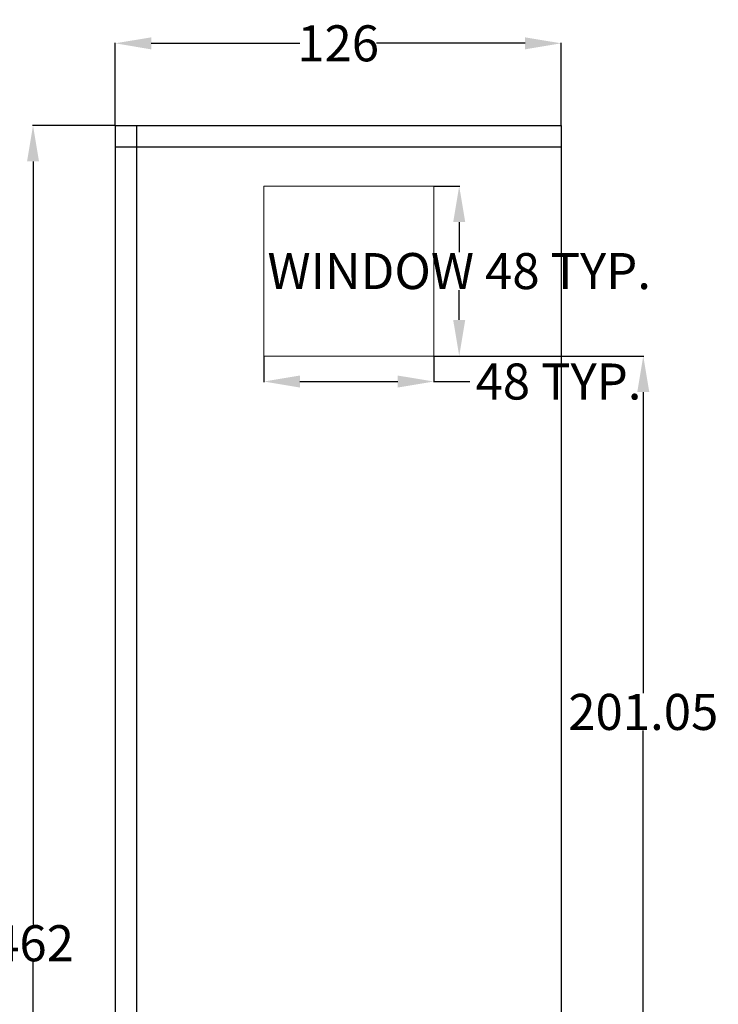
# Model space of a CAD drawing. Units: inches. Extents: x -107 to 647, y -210 to 500.
# Tile 7 of 7: x 450 to 647, y 216 to 494. Entities that reach past the tile are written whole.
import ezdxf

# ---------------------------------------------------------------- set-up
doc = ezdxf.new("R2010")
doc.units = ezdxf.units.IN
doc.header["$MEASUREMENT"] = 0
for name, color, linetype, lineweight in [('A-ANNO-DIMS', 2, 'Continuous', 18), ('A-ELEV', 30, 'Continuous', 25), ('A-ELEV-GLAZ', 4, 'Continuous', 18)]:
    doc.layers.add(name, color=color, linetype=linetype, lineweight=lineweight)
doc.styles.get("Standard").update_dxf_attribs({"font": 'arial.ttf'})
doc.dimstyles.get("Standard").update_dxf_attribs({"dimtxt": 10.18, "dimasz": 10.18, "dimexe": 0.18, "dimexo": 0.0625, "dimgap": 0.09, "dimtad": 0, "dimtih": 1, "dimtoh": 1, "dimdec": 0, "dimzin": 0, "dimdsep": 46, "dimlunit": 3, "dimtxsty": 'Standard', "dimcen": 0.09, "dimadec": 0, "dimazin": 0, "dimtfac": 1, "dimtdec": 0, "dimtofl": 0, "dimtmove": 0, "dimatfit": 3, "dimfxl": 1, "dimtolj": 1, "dimtzin": 0, "dimarcsym": 0})

# ---------------------------------------------------------------- blocks, each defined once
blk = doc.blocks.new('WINDOW-ELEV-48X48IN')
blk.add_lwpolyline([(0, 48), (48, 48), (48, 0), (0, 0)], close=True)
blk = doc.blocks.new('*D42')
at = {"layer": 'A-ANNO-DIMS', "color": 0, "lineweight": -2, "transparency": 16777216}
for p, q in [((566.81, 447.2), (574.13, 447.2)), ((573.95, 437.02), (573.95, 428.55)), ((573.95, 409.38), (573.95, 417.84)), ((566.81, 399.2), (574.13, 399.2))]:
    blk.add_line(p, q, dxfattribs=at)
at = {"layer": 'A-ANNO-DIMS', "color": 0, "transparency": 16777216}
for points in [[(572.25, 437.02), (575.65, 437.02), (573.95, 447.2)], [(572.25, 409.38), (575.65, 409.38), (573.95, 399.2)]]:
    blk.add_solid(points, dxfattribs=at)
at = {"layer": 'Defpoints', "color": 0, "transparency": 16777216}
for p in [(566.75, 447.2), (573.95, 447.2), (566.75, 399.2)]:
    blk.add_point(p, dxfattribs=at)
at = {"layer": 'A-ANNO-DIMS', "color": 0, "transparency": 16777216, "insert": (573.95, 423.2), "char_height": 10.18, "attachment_point": 5}
blk.add_mtext('\\A1;WINDOW 48 TYP.', dxfattribs=at)
blk = doc.blocks.new('*D43')
at = {"layer": 'A-ANNO-DIMS', "color": 0, "lineweight": -2, "transparency": 16777216}
for p, q in [((518.75, 399.14), (518.75, 391.82)), ((566.75, 399.14), (566.75, 391.82)), ((528.93, 392), (556.57, 392)), ((566.75, 392), (576.93, 392))]:
    blk.add_line(p, q, dxfattribs=at)
at = {"layer": 'A-ANNO-DIMS', "color": 0, "transparency": 16777216}
for points in [[(528.93, 393.69), (528.93, 390.3), (518.75, 392)], [(556.57, 393.69), (556.57, 390.3), (566.75, 392)]]:
    blk.add_solid(points, dxfattribs=at)
at = {"layer": 'Defpoints', "color": 0, "transparency": 16777216}
for p in [(518.75, 399.2), (566.75, 399.2), (566.75, 392)]:
    blk.add_point(p, dxfattribs=at)
at = {"layer": 'A-ANNO-DIMS', "color": 0, "transparency": 16777216, "insert": (602, 392), "char_height": 10.18, "attachment_point": 5}
blk.add_mtext('\\A1;48 TYP.', dxfattribs=at)
blk = doc.blocks.new('*D98')
at = {"layer": 'A-ANNO-DIMS', "color": 0, "lineweight": -2, "transparency": 16777216}
for p, q in [((476.69, 464.33), (453.37, 464.33)), ((453.55, 454.15), (453.55, 238.61)), ((453.55, 12.51), (453.55, 228.04)), ((476.69, 2.33), (453.37, 2.33))]:
    blk.add_line(p, q, dxfattribs=at)
at = {"layer": 'A-ANNO-DIMS', "color": 0, "transparency": 16777216}
for points in [[(451.85, 454.15), (455.25, 454.15), (453.55, 464.33)], [(451.85, 12.51), (455.25, 12.51), (453.55, 2.33)]]:
    blk.add_solid(points, dxfattribs=at)
at = {"layer": 'Defpoints', "color": 0, "transparency": 16777216}
for p in [(453.55, 464.33), (476.75, 464.33), (476.75, 2.33)]:
    blk.add_point(p, dxfattribs=at)
at = {"layer": 'A-ANNO-DIMS', "color": 0, "transparency": 16777216, "insert": (453.55, 233.33), "char_height": 10.18, "attachment_point": 5}
blk.add_mtext('\\A1;462', dxfattribs=at)
blk = doc.blocks.new('*D99')
at = {"layer": 'A-ANNO-DIMS', "color": 0, "lineweight": -2, "transparency": 16777216}
for p, q in [((476.75, 464.39), (476.75, 487.71)), ((486.93, 487.53), (528.9, 487.53)), ((592.57, 487.53), (550.6, 487.53)), ((602.75, 464.39), (602.75, 487.71))]:
    blk.add_line(p, q, dxfattribs=at)
at = {"layer": 'A-ANNO-DIMS', "color": 0, "transparency": 16777216}
for points in [[(486.93, 489.22), (486.93, 485.83), (476.75, 487.53)], [(592.57, 489.22), (592.57, 485.83), (602.75, 487.53)]]:
    blk.add_solid(points, dxfattribs=at)
at = {"layer": 'Defpoints', "color": 0, "transparency": 16777216}
for p in [(602.75, 487.53), (476.75, 464.33), (602.75, 464.33)]:
    blk.add_point(p, dxfattribs=at)
at = {"layer": 'A-ANNO-DIMS', "color": 0, "transparency": 16777216, "insert": (539.75, 487.53), "char_height": 10.18, "attachment_point": 5}
blk.add_mtext('\\A1;126', dxfattribs=at)
blk = doc.blocks.new('*D101')
at = {"layer": 'A-ANNO-DIMS', "color": 0, "lineweight": -2, "transparency": 16777216}
for p, q in [((566.81, 399.2), (626.13, 399.2)), ((625.95, 389.02), (625.95, 303.96)), ((625.95, 208.33), (625.95, 293.39)), ((566.81, 198.15), (626.13, 198.15))]:
    blk.add_line(p, q, dxfattribs=at)
at = {"layer": 'A-ANNO-DIMS', "color": 0, "transparency": 16777216}
for points in [[(624.25, 389.02), (627.65, 389.02), (625.95, 399.2)], [(624.25, 208.33), (627.65, 208.33), (625.95, 198.15)]]:
    blk.add_solid(points, dxfattribs=at)
at = {"layer": 'Defpoints', "color": 0, "transparency": 16777216}
for p in [(566.75, 399.2), (625.95, 399.2), (566.75, 198.15)]:
    blk.add_point(p, dxfattribs=at)
at = {"layer": 'A-ANNO-DIMS', "color": 0, "transparency": 16777216, "insert": (625.95, 298.67), "char_height": 10.18, "attachment_point": 5}
blk.add_mtext('\\A1;201.05', dxfattribs=at)

msp = doc.modelspace()

# ---------------------------------------------------------------- linework, layer by layer
at = {"layer": 'A-ELEV'}
for p, q in [((476.749, 464.325), (476.749, 2.325)), ((476.749, 464.325), (602.749, 464.325)), ((482.749, 464.325), (482.749, 2.325)), ((602.749, 464.325), (602.749, 2.325)), ((476.749, 458.325), (602.749, 458.325))]:
    msp.add_line(p, q, dxfattribs=at)

# ---------------------------------------------------------------- block references
at = {"layer": 'A-ELEV-GLAZ'}
msp.add_blockref('WINDOW-ELEV-48X48IN', (518.749, 399.198), dxfattribs=at)

# ---------------------------------------------------------------- dimensions: what is measured, and where the dimension line sits
at = {"layer": 'A-ANNO-DIMS'}
dim = msp.add_linear_dim(base=(602.749, 487.525), p1=(476.749, 464.325), p2=(602.749, 464.325), dimstyle='Standard', override={"dimdec": 0, "dimlfac": 1, "dimrnd": 0, "dimzin": 0, "dimdsep": 46, "dimlunit": 2}, dxfattribs=at)
dim.commit()
dim.dimension.update_dxf_attribs({"geometry": '*D99', "text_midpoint": (539.749, 487.525)})
for base, p1, p2, override, picture, middle in [((453.549, 464.325), (476.749, 2.325), (476.749, 464.325), {"dimdec": 0, "dimlfac": 1, "dimrnd": 0, "dimzin": 0, "dimdsep": 46, "dimlunit": 2}, '*D98', (453.549, 233.325)), ((625.949, 399.198), (566.749, 198.148), (566.749, 399.198), {"dimdec": 2, "dimlfac": 1, "dimrnd": 0, "dimzin": 0, "dimdsep": 46, "dimlunit": 2}, '*D101', (625.949, 298.673))]:
    dim = msp.add_linear_dim(base=base, p1=p1, p2=p2, angle=90, dimstyle='Standard', override=override, dxfattribs=at)
    dim.commit()
    dim.dimension.update_dxf_attribs({"geometry": picture, "text_midpoint": middle})
dim = msp.add_linear_dim(base=(573.949, 447.198), p1=(566.749, 399.198), p2=(566.749, 447.198), angle=90, text='WINDOW <> TYP.', dimstyle='Standard', override={"dimdec": 0, "dimlfac": 1, "dimrnd": 0, "dimzin": 0, "dimdsep": 46, "dimlunit": 2}, dxfattribs=at)
dim.commit()
dim.dimension.update_dxf_attribs({"geometry": '*D42', "text_midpoint": (573.949, 423.198)})
dim = msp.add_linear_dim(base=(566.749, 391.998), p1=(518.749, 399.198), p2=(566.749, 399.198), text='<> TYP.', dimstyle='Standard', override={"dimdec": 0, "dimlfac": 1, "dimrnd": 0, "dimzin": 0, "dimdsep": 46, "dimlunit": 2}, dxfattribs=at)
dim.commit()
dim.dimension.update_dxf_attribs({"geometry": '*D43', "text_midpoint": (602, 391.998)})

doc.saveas('drawing.dxf')
